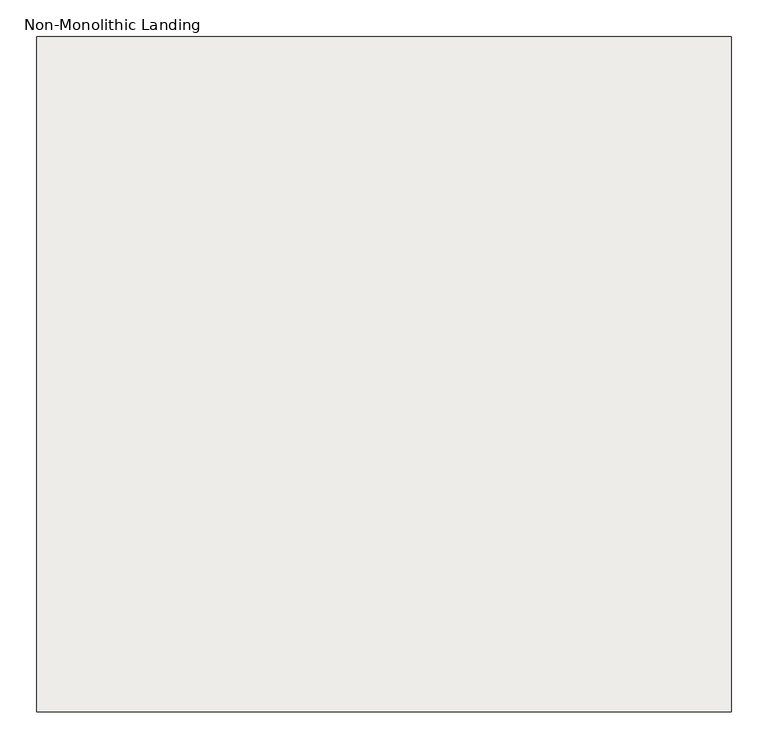
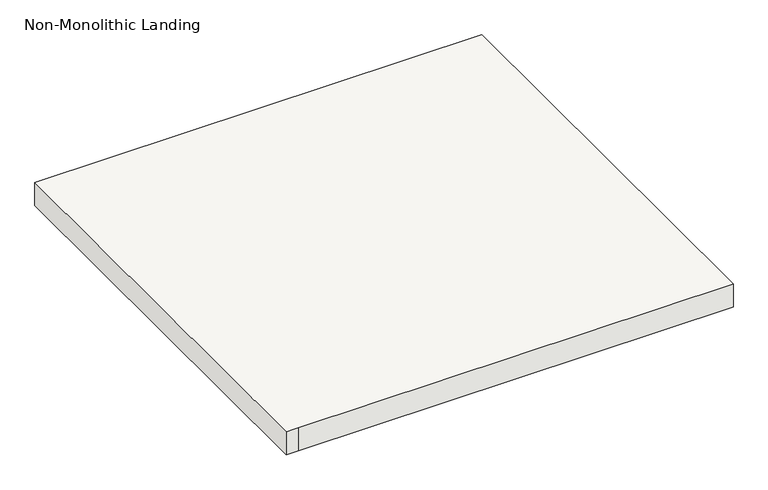
"""IFC4 building model written with IfcOpenShell, lengths in millimetres: slab geometry, Non-Monolithic Landing."""

from ifc_helpers import new_model, si_unit, origin, place, context, project, spatial, faceted_brep, source, transform, mapped, element, save


def non_monolithic_landing_8c0399ef(model_context):
    return source(origin(), model_context, "Body", "Brep", [
        faceted_brep([(111.2391502, 2117.5115866, 5230.2833333), (111.2391502, 2092.1115866, 5204.8833333), (-803.1608498, 2092.1115866, 5204.8833333), (-803.1608498, 2117.5115866, 5230.2833333), (-828.5608498, 2117.5115866, 5249.3333333), (-828.5608498, 1203.1115866, 5249.3333333), (-803.1608498, 1203.1115866, 5249.3333333), (111.2391502, 1203.1115866, 5249.3333333), (111.2391502, 2117.5115866, 5249.3333333), (-803.1608498, 2092.1115866, 5198.5333333), (111.2391502, 2092.1115866, 5198.5333333), (111.2391502, 1203.1115866, 5198.5333333), (-803.1608498, 1203.1115866, 5198.5333333), (-828.5608498, 1203.1115866, 5198.5333333), (-828.5608498, 2117.5115866, 5198.5333333), (-803.1608498, 2117.5115866, 5198.5333333)], [[[0, 1, 2, 3]], [[4, 5, 6, 7, 8]], [[9, 10, 11, 12, 13, 14, 15]], [[10, 9, 2, 1]], [[9, 15, 3, 2]], [[4, 8, 0, 3, 15, 14]], [[5, 4, 14, 13]], [[6, 5, 13, 12]], [[7, 6, 12, 11]], [[8, 7, 11, 10, 1, 0]]]),
    ])


if __name__ == "__main__":
    model = new_model("IFC4")
    model_context = context("Model", 3, world=origin())
    ifc_project = project(units=[si_unit("LENGTHUNIT", "METRE", prefix="MILLI")], contexts=[model_context])
    site = spatial("IfcSite", under=ifc_project)
    building = spatial("IfcBuilding", under=site)
    placement = place(None, origin())
    non_monolithic_landing_shape = non_monolithic_landing_8c0399ef(model_context)
    element("IfcSlab", 1, ObjectType="Non-Monolithic Landing", at=placement, inside=building, context=model_context, shape_type="MappedRepresentation", body=[
        mapped(non_monolithic_landing_shape, transform((0.0, 0.0, 0.0), x_axis=(1.0, 0.0, 0.0), y_axis=(0.0, 1.0, 0.0), z_axis=(0.0, 0.0, 1.0))),
    ])
    save(model, "model.ifc")
